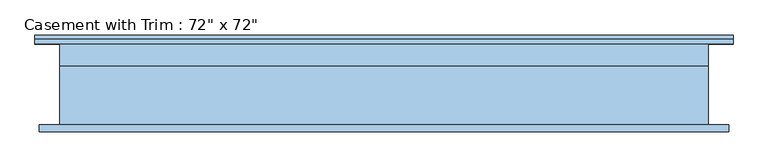
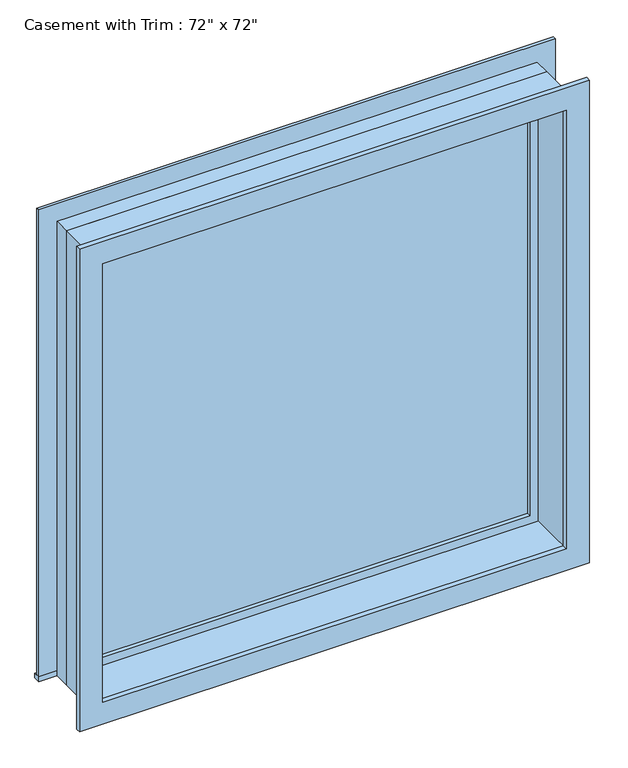
"""IFC4 building model written with IfcOpenShell, lengths in millimetres: window geometry."""

from ifc_helpers import new_model, si_unit, frame, origin, place, context, project, spatial, polyline, outline, extrude, source, transform, mapped, element, save


def window_4294005a(model_context):
    return source(origin(), model_context, "Body", "SweptSolid", [
        extrude(outline(polyline([(-984.25, 139.7), (984.25, 139.7), (984.25, 114.3), (-984.25, 114.3), (-984.25, 139.7)])), frame((0.0, 0.0, 609.6), z_axis=(0.0, 0.0, 1.0), x_axis=(1.0, 0.0, 0.0)), (0.0, 0.0, 1.0), 19.05),
        extrude(outline(polyline([(2419.35, -895.35), (2419.35, 895.35), (628.65, 895.35), (628.65, 984.25), (2508.25, 984.25), (2508.25, -984.25), (628.65, -984.25), (628.65, -895.35), (2419.35, -895.35)])), frame((0.0, 114.3, 0.0), z_axis=(0.0, 1.0, 0.0), x_axis=(0.0, 0.0, 1.0)), (0.0, 0.0, 1.0), 12.7),
        extrude(outline(polyline([(2495.55, 971.55), (2495.55, -971.55), (552.45, -971.55), (552.45, 971.55), (2495.55, 971.55)]), holes=[polyline([(2406.65, 882.65), (641.35, 882.65), (641.35, -882.65), (2406.65, -882.65), (2406.65, 882.65)])]), frame((0.0, -133.35, 0.0), z_axis=(0.0, 1.0, 0.0), x_axis=(0.0, 0.0, 1.0)), (0.0, 0.0, 1.0), 19.05),
        extrude(outline(polyline([(850.9, 66.675), (-850.9, 66.675), (-850.9, 79.375), (850.9, 79.375), (850.9, 66.675)])), frame((0.0, 0.0, 673.1), z_axis=(0.0, 0.0, 1.0), x_axis=(1.0, 0.0, 0.0)), (0.0, 0.0, 1.0), 1701.8),
        extrude(outline(polyline([(2419.35, -895.35), (628.65, -895.35), (628.65, 895.35), (2419.35, 895.35), (2419.35, -895.35)]), holes=[polyline([(2374.9, -850.9), (2374.9, 850.9), (673.1, 850.9), (673.1, -850.9), (2374.9, -850.9)])]), frame((0.0, 50.8, 0.0), z_axis=(0.0, 1.0, 0.0), x_axis=(0.0, 0.0, 1.0)), (0.0, 0.0, 1.0), 44.45),
        extrude(outline(polyline([(2438.4, -914.4), (609.6, -914.4), (609.6, 914.4), (2438.4, 914.4), (2438.4, -914.4)]), holes=[polyline([(2406.65, -882.65), (2406.65, 882.65), (641.35, 882.65), (641.35, -882.65), (2406.65, -882.65)])]), frame((0.0, -114.3, 0.0), z_axis=(0.0, 1.0, 0.0), x_axis=(0.0, 0.0, 1.0)), (0.0, 0.0, 1.0), 165.1),
        extrude(outline(polyline([(2438.4, 914.4), (2438.4, -914.4), (609.6, -914.4), (609.6, 914.4), (2438.4, 914.4)]), holes=[polyline([(2419.35, 895.35), (628.65, 895.35), (628.65, -895.35), (2419.35, -895.35), (2419.35, 895.35)])]), frame((0.0, 50.8, 0.0), z_axis=(0.0, 1.0, 0.0), x_axis=(0.0, 0.0, 1.0)), (0.0, 0.0, 1.0), 63.5),
    ])


if __name__ == "__main__":
    model = new_model("IFC4")
    model_context = context("Model", 3, world=origin())
    ifc_project = project(units=[si_unit("LENGTHUNIT", "METRE", prefix="MILLI")], contexts=[model_context])
    site = spatial("IfcSite", under=ifc_project)
    building = spatial("IfcBuilding", under=site)
    placement = place(None, origin())
    window_shape = window_4294005a(model_context)
    element("IfcWindow", 1, ObjectType="Casement with Trim : 72\" x 72\"", at=placement, inside=building, context=model_context, shape_type="MappedRepresentation", body=[
        mapped(window_shape, transform((0.0, 0.0, 0.0), x_axis=(1.0, 0.0, 0.0), y_axis=(0.0, 1.0, 0.0), z_axis=(0.0, 0.0, 1.0))),
    ])
    save(model, "model.ifc")

# Revit data of these elements
# Type "Casement with Trim : 72\" x 72\""
#   Type Mark = "18"
#   Construction Type Id = "GSP4R"
#   Assembly Code = "B2020100"
#   Analytic Construction = "1/8 in Pilkington single glazing"
#   Visual Light Transmittance = 0.9
#   Solar Heat Gain Coefficient = 0.78
#   Heat Transfer Coefficient (U) = 0.6496 BTU/(h·ft²·°F)
#   Height = 6' - 0"
#   Default Sill Height = 2' - 0"
#   Trim Projection - Ext. = 0' - 0 1/2"
#   Trim Projection - Int. = 0' - 0 3/4"
#   Trim Width - Exterior = 0' - 3 1/2"
#   Trim Width - Interior = 0' - 3 1/2"
#   Width = 6' - 0"
#   Window Inset = 0' - 0 3/4"
#   Define Thermal Properties by = 1
#   Glass Pane Material = Glass
#   Sash Material = Stainless Steel
#   Trim Exterior Material = Stainless Steel
#   Trim Interior Material = Steel, Polished
#   Wall Closure = (empty or 0)
# Element 1 (IfcWindow, "Casement with Trim : 72\" x 72\"")
#   Materials on its faces: "Stainless Steel", "Steel, Polished", "Glass"
# Materials
#   "Glass": class "Glass", colour RGB 0 128 192, transparency 0.75, Description = "Soda Lime Glass", Cost = 0
#   "Stainless Steel": class "Metal", colour RGB 0 0 0, transparency 0, Description = "Stainless Steel 18/8", Cost = 0
#   "Steel, Polished": class "Metal", colour RGB 57 57 57, transparency 0, Description = "Polished steel", Cost = 0
